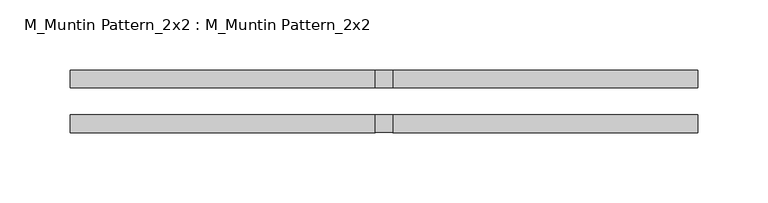
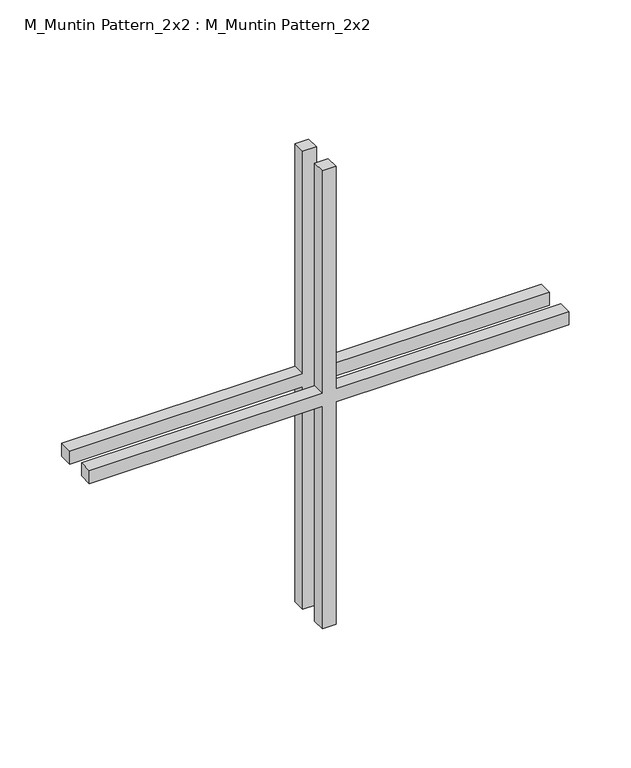
"""IFC4 building model written with IfcOpenShell, lengths in millimetres: proxy geometry, M_Muntin Pattern_2x2 : M_Muntin Pattern_2x2."""

from ifc_helpers import new_model, si_unit, frame, origin, place, context, project, spatial, polyline, outline, extrude, source, transform, mapped, element, save


def m_muntin_pattern_2x2_m_muntin_pattern_2x2_6483b455(model_context):
    return source(origin(), model_context, "Body", "SweptSolid", [
        extrude(outline(polyline([(232.1375, -6.35), (232.1375, -223.8), (219.4375, -223.8), (219.4375, -6.35), (0.0, -6.35), (0.0, 6.35), (219.4375, 6.35), (219.4375, 223.8), (232.1375, 223.8), (232.1375, 6.35), (451.575, 6.35), (451.575, -6.35), (232.1375, -6.35)])), frame((0.0, 9.525, 0.0), z_axis=(0.0, 1.0, 0.0), x_axis=(0.0, 0.0, 1.0)), (0.0, 0.0, 1.0), 12.7),
        extrude(outline(polyline([(232.1375, -6.35), (232.1375, -223.8), (219.4375, -223.8), (219.4375, -6.35), (0.0, -6.35), (0.0, 6.35), (219.4375, 6.35), (219.4375, 223.8), (232.1375, 223.8), (232.1375, 6.35), (451.575, 6.35), (451.575, -6.35), (232.1375, -6.35)])), frame((0.0, -22.225, 0.0), z_axis=(0.0, 1.0, 0.0), x_axis=(0.0, 0.0, 1.0)), (0.0, 0.0, 1.0), 12.7),
    ])


if __name__ == "__main__":
    model = new_model("IFC4")
    model_context = context("Model", 3, world=origin())
    ifc_project = project(units=[si_unit("LENGTHUNIT", "METRE", prefix="MILLI")], contexts=[model_context])
    site = spatial("IfcSite", under=ifc_project)
    building = spatial("IfcBuilding", under=site)
    placement = place(None, origin())
    m_muntin_pattern_2x2_m_muntin_pattern_2x2_shape = m_muntin_pattern_2x2_m_muntin_pattern_2x2_6483b455(model_context)
    element("IfcBuildingElementProxy", 1, Name="M_Muntin Pattern_2x2 : M_Muntin Pattern_2x2", ObjectType="M_Muntin Pattern_2x2 : M_Muntin Pattern_2x2", at=placement, inside=building, context=model_context, shape_type="MappedRepresentation", body=[
        mapped(m_muntin_pattern_2x2_m_muntin_pattern_2x2_shape, transform((0.0, 0.0, 0.0), x_axis=(1.0, 0.0, 0.0), y_axis=(0.0, 1.0, 0.0), z_axis=(0.0, 0.0, 1.0))),
    ])
    save(model, "model.ifc")

# Revit data of these elements
# Type "M_Muntin Pattern_2x2 : M_Muntin Pattern_2x2"
#   Width [instance default] = 1.2 m
#   Thickness = 0.0127 m
#   Height [instance default] = 1.2 m
#   Distance = 0.01905 m
#   Interior Material [instance default] = none
#   Exterior Material [instance default] = none
#   Default Elevation = 0
# Element 1 (IfcBuildingElementProxy, "M_Muntin Pattern_2x2 : M_Muntin Pattern_2x2")
#   Width = 0.4476 m
#   Height = 0.451575 m
#   Interior Material = Wood - Stained
#   Exterior Material = Clad - White
#   Materials on its faces: "Clad - White", "Wood - Stained"
# Materials
#   "Clad - White": class "Wood", colour RGB 242 242 238, transparency 0, Cost = 0
#   "Wood - Stained": class "Wood", colour RGB 224 178 126, transparency 0, Cost = 0
